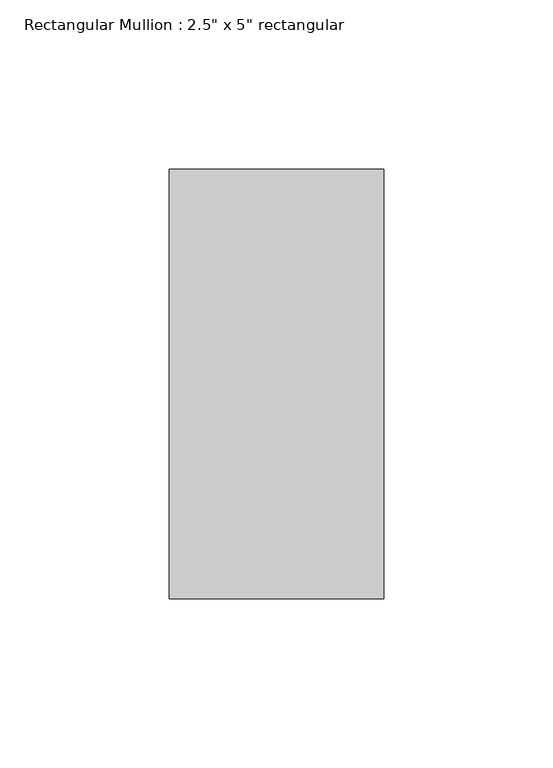
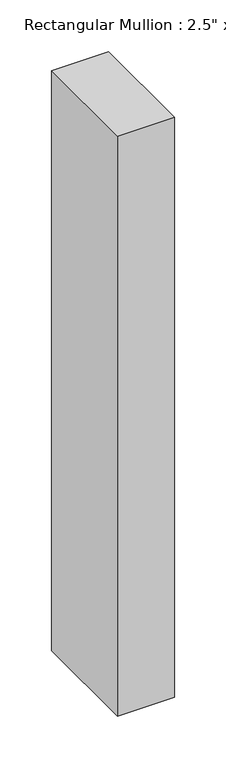
"""IFC4 building model written with IfcOpenShell, lengths in millimetres: member geometry."""

from ifc_helpers import new_model, si_unit, frame, origin, place, context, project, spatial, polyline, outline, extrude, source, transform, mapped, element, save


def member_aebd74a6(model_context):
    return source(origin(), model_context, "Body", "SweptSolid", [
        extrude(outline(polyline([(31.75, 63.5), (31.75, -63.5), (-31.75, -63.5), (-31.75, 63.5), (31.75, 63.5)])), frame((0.0, 0.0, -683.6567525), z_axis=(0.0, 0.0, 1.0), x_axis=(1.0, 0.0, 0.0)), (0.0, 0.0, 1.0), 683.6567525),
    ])


if __name__ == "__main__":
    model = new_model("IFC4")
    model_context = context("Model", 3, world=origin())
    ifc_project = project(units=[si_unit("LENGTHUNIT", "METRE", prefix="MILLI")], contexts=[model_context])
    site = spatial("IfcSite", under=ifc_project)
    building = spatial("IfcBuilding", under=site)
    placement = place(None, origin())
    member_shape = member_aebd74a6(model_context)
    element("IfcMember", 1, ObjectType="Rectangular Mullion : 2.5\" x 5\" rectangular", at=placement, inside=building, context=model_context, shape_type="MappedRepresentation", body=[
        mapped(member_shape, transform((0.0, 0.0, 0.0), x_axis=(1.0, 0.0, 0.0), y_axis=(0.0, 1.0, 0.0), z_axis=(0.0, 0.0, 1.0))),
    ])
    save(model, "model.ifc")

# Revit data of these elements
# Type "Rectangular Mullion : 2.5\" x 5\" rectangular"
#   built-in parameter 1007304 = 0.416667 (stored number, unit not read)
#   built-in parameter 1007301 = 0.104167 (stored number, unit not read)
#   built-in parameter 1007300 = 0.104167 (stored number, unit not read)
# Element 1 (IfcMember, "Rectangular Mullion : 2.5\" x 5\" rectangular")
#   Materials on its faces: "Aluminum"
# Materials
#   "Aluminum": class "Metal", colour RGB 247 247 247, transparency 0, Description = "Aluminum 6061", Cost = 0
